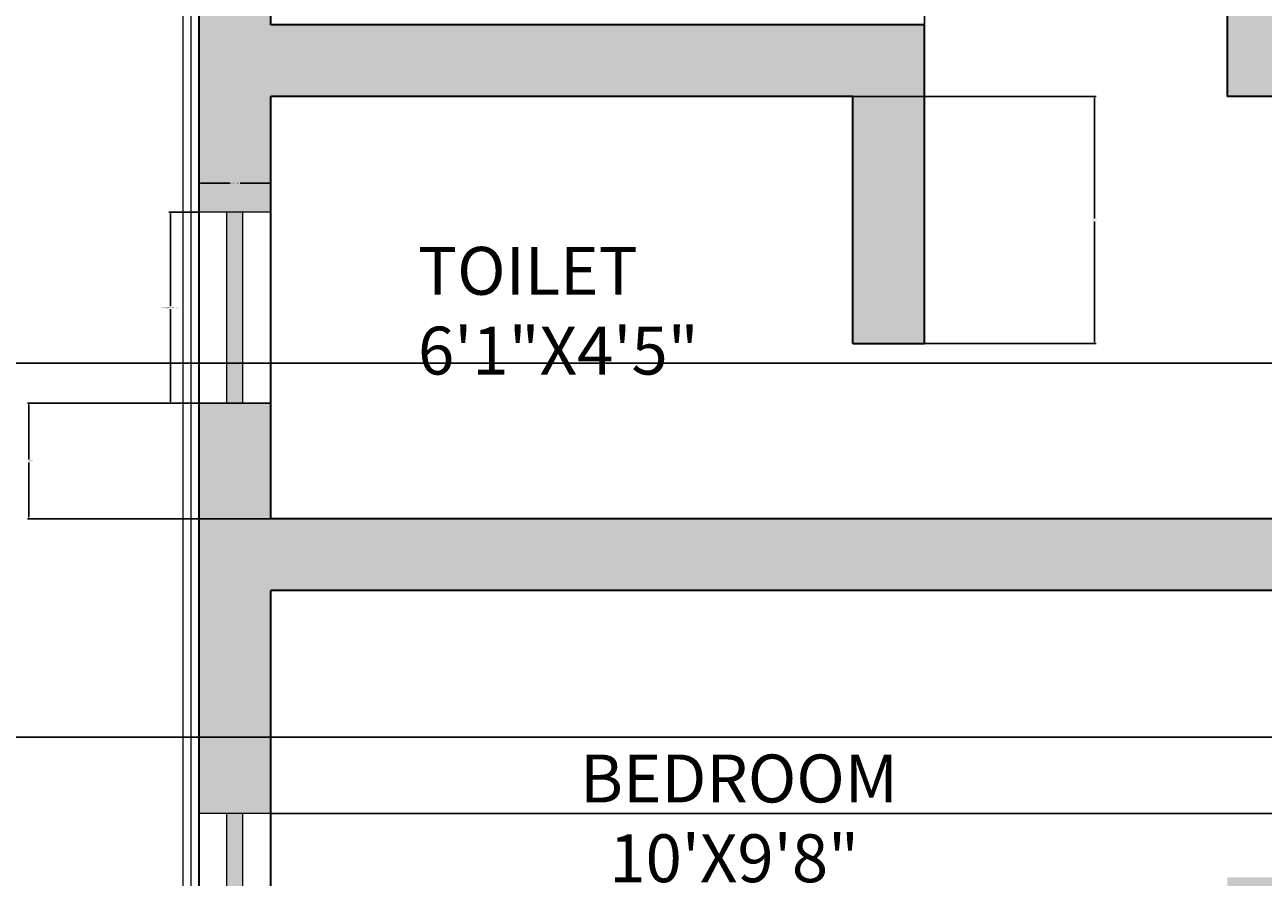
# Model space of a CAD drawing. Units: inches. Extents: x 311 to 815, y -527 to 136.
# Tile 16 of 21: x 388 to 544, y -210 to -103. Entities that reach past the tile are written whole.
import ezdxf

# ---------------------------------------------------------------- set-up
doc = ezdxf.new("R2010")
doc.units = ezdxf.units.IN
doc.header["$MEASUREMENT"] = 0
for name, color, linetype, lineweight in [('A-ANNO-DIMS', 1, 'Continuous', 18), ('A-AREA-IDEN', 8, 'Continuous', 18), ('A-FLOR-EDGE', 1, 'Continuous', 18), ('A-GLAZ-PATT', 5, 'Continuous', 13), ('A-WALL-PATT', 242, 'Continuous', 13), ('wall', 1, 'Continuous', 35), ('win', 5, 'Continuous', 18)]:
    doc.layers.add(name, color=color, linetype=linetype, lineweight=lineweight)
doc.styles.get("Standard").update_dxf_attribs({"font": 'arial.ttf'})
doc.dimstyles.get("Standard").update_dxf_attribs({"dimtxt": 0.18, "dimasz": 0.18, "dimexe": 0.18, "dimexo": 0.0625, "dimgap": 0.09, "dimtad": 0, "dimtih": 1, "dimtoh": 1, "dimdec": 1, "dimzin": 0, "dimdsep": 46, "dimlunit": 4, "dimtxsty": 'Standard', "dimcen": 0.09, "dimadec": 0, "dimazin": 0, "dimtfac": 1, "dimtdec": 1, "dimtofl": 0, "dimtmove": 0, "dimatfit": 3, "dimfxl": 1, "dimtolj": 1, "dimtzin": 0, "dimarcsym": 0})

# ---------------------------------------------------------------- blocks, each defined once
blk = doc.blocks.new('_ArchTick')
at = {"color": 0, "linetype": 'ByBlock', "const_width": 0.15}
blk.add_lwpolyline([(-0.5, -0.5), (0.5, 0.5)], dxfattribs=at)
blk = doc.blocks.new('_Oblique')
at = {"color": 0, "linetype": 'ByBlock', "lineweight": -2}
blk.add_line((-0.5, -0.5), (0.5, 0.5), dxfattribs=at)
blk = doc.blocks.new('*D3')
at = {"layer": 'A-ANNO-DIMS', "color": 0, "lineweight": -2, "transparency": 16777216}
for p, q in [((377.54, 21.87), (377.54, -221.61)), ((377.54, -482.13), (377.54, -238.65))]:
    blk.add_line(p, q, dxfattribs=at)
at = {"layer": 'Defpoints', "color": 0, "transparency": 16777216}
for p in [(410.32, 21.87), (377.54, -482.13), (410.32, -482.13)]:
    blk.add_point(p, dxfattribs=at)
at = {"layer": 'A-ANNO-DIMS', "color": 0, "lineweight": -2, "transparency": 16777216, "xscale": 9, "yscale": 9, "zscale": 9}
for name, p, rotation in [('_ArchTick', (377.54, 21.87), 90), ('_Oblique', (377.54, -482.13), 270)]:
    blk.add_blockref(name, p, dxfattribs=dict(at, rotation=rotation))
at = {"layer": 'A-ANNO-DIMS', "color": 0, "transparency": 16777216, "insert": (377.54, -230.13), "char_height": 9, "attachment_point": 5}
blk.add_mtext("\\A1;42'", dxfattribs=at)
blk = doc.blocks.new('WIN-60IN')
for p, q in [((9, 60), (0, 60)), ((3.5, 0), (3.5, 60)), ((5.5, 0), (5.5, 60)), ((9, 0), (0, 0))]:
    blk.add_line(p, q)
blk = doc.blocks.new('WIN-24IN')
for p, q in [((9, 24), (0, 24)), ((3.5, 0), (3.5, 24)), ((5.5, 0), (5.5, 24)), ((9, 0), (0, 0))]:
    blk.add_line(p, q)
blk = doc.blocks.new('*D12')
at = {"layer": 'A-ANNO-DIMS', "color": 0, "lineweight": -2, "transparency": 16777216}
for p, q in [((410.26, -126.63), (406.54, -126.63)), ((406.72, -126.81), (406.72, -138.44)), ((406.72, -150.45), (406.72, -138.81)), ((410.26, -150.63), (406.54, -150.63))]:
    blk.add_line(p, q, dxfattribs=at)
at = {"layer": 'A-ANNO-DIMS', "color": 0, "transparency": 16777216}
for points in [[(406.69, -126.81), (406.75, -126.81), (406.72, -126.63)], [(406.69, -150.45), (406.75, -150.45), (406.72, -150.63)]]:
    blk.add_solid(points, dxfattribs=at)
at = {"layer": 'Defpoints', "color": 0, "transparency": 16777216}
for p in [(406.72, -126.63), (410.32, -126.63), (410.32, -150.63)]:
    blk.add_point(p, dxfattribs=at)
at = {"layer": 'A-ANNO-DIMS', "color": 0, "transparency": 16777216, "insert": (406.72, -138.63), "char_height": 0.18, "attachment_point": 5}
blk.add_mtext('\\A1;WINDOW 2\'-0" TYP.', dxfattribs=at)
blk = doc.blocks.new('*D13')
at = {"layer": 'A-ANNO-DIMS', "color": 0, "lineweight": -2, "transparency": 16777216}
for p, q in [((410.32, -126.57), (410.32, -122.85)), ((410.5, -123.03), (414.18, -123.03)), ((419.14, -123.03), (415.46, -123.03)), ((419.32, -126.57), (419.32, -122.85))]:
    blk.add_line(p, q, dxfattribs=at)
at = {"layer": 'A-ANNO-DIMS', "color": 0, "transparency": 16777216}
for points in [[(410.5, -123), (410.5, -123.06), (410.32, -123.03)], [(419.14, -123), (419.14, -123.06), (419.32, -123.03)]]:
    blk.add_solid(points, dxfattribs=at)
at = {"layer": 'Defpoints', "color": 0, "transparency": 16777216}
for p in [(419.32, -123.03), (410.32, -126.63), (419.32, -126.63)]:
    blk.add_point(p, dxfattribs=at)
at = {"layer": 'A-ANNO-DIMS', "color": 0, "transparency": 16777216, "insert": (414.82, -123.03), "char_height": 0.18, "attachment_point": 5}
blk.add_mtext('\\A1;0\'-9" TYP.', dxfattribs=at)
blk = doc.blocks.new('*D32')
at = {"layer": 'A-ANNO-DIMS', "color": 0, "lineweight": -2, "transparency": 16777216}
for p, q in [((671.64, -145.62), (377.79, -145.62)), ((377.97, -145.8), (377.97, -168.9)), ((377.97, -192.37), (377.97, -169.27)), ((671.64, -192.55), (377.79, -192.55))]:
    blk.add_line(p, q, dxfattribs=at)
at = {"layer": 'A-ANNO-DIMS', "color": 0, "transparency": 16777216}
for points in [[(377.94, -145.8), (378, -145.8), (377.97, -145.62)], [(377.94, -192.37), (378, -192.37), (377.97, -192.55)]]:
    blk.add_solid(points, dxfattribs=at)
at = {"layer": 'Defpoints', "color": 0, "transparency": 16777216}
for p in [(671.7, -145.62), (377.97, -192.55), (671.7, -192.55)]:
    blk.add_point(p, dxfattribs=at)
at = {"layer": 'A-ANNO-DIMS', "color": 0, "transparency": 16777216, "insert": (377.97, -169.08), "char_height": 0.18, "attachment_point": 5}
blk.add_mtext('\\A1;3\'-11"', dxfattribs=at)
blk = doc.blocks.new('*D41')
at = {"layer": 'A-ANNO-DIMS', "color": 0, "lineweight": -2, "transparency": 16777216}
for p, q in [((419.26, -150.63), (388.79, -150.63)), ((388.97, -150.81), (388.97, -157.69)), ((388.97, -164.95), (388.97, -158.06)), ((419.26, -165.13), (388.79, -165.13))]:
    blk.add_line(p, q, dxfattribs=at)
at = {"layer": 'A-ANNO-DIMS', "color": 0, "transparency": 16777216}
for points in [[(388.94, -150.81), (389, -150.81), (388.97, -150.63)], [(388.94, -164.95), (389, -164.95), (388.97, -165.13)]]:
    blk.add_solid(points, dxfattribs=at)
at = {"layer": 'Defpoints', "color": 0, "transparency": 16777216}
for p in [(388.97, -150.63), (419.32, -150.63), (419.32, -165.13)]:
    blk.add_point(p, dxfattribs=at)
at = {"layer": 'A-ANNO-DIMS', "color": 0, "transparency": 16777216, "insert": (388.97, -157.88), "char_height": 0.18, "attachment_point": 5}
blk.add_mtext('\\A1;1\'-2 1/2"', dxfattribs=at)
blk = doc.blocks.new('*D42')
at = {"layer": 'A-ANNO-DIMS', "color": 0, "lineweight": -2, "transparency": 16777216}
for p, q in [((419.39, -174.13), (754.85, -174.13)), ((754.67, -174.31), (754.67, -187.95)), ((754.67, -201.95), (754.67, -188.31)), ((419.39, -202.13), (754.85, -202.13))]:
    blk.add_line(p, q, dxfattribs=at)
at = {"layer": 'A-ANNO-DIMS', "color": 0, "transparency": 16777216}
for points in [[(754.64, -174.31), (754.7, -174.31), (754.67, -174.13)], [(754.64, -201.95), (754.7, -201.95), (754.67, -202.13)]]:
    blk.add_solid(points, dxfattribs=at)
at = {"layer": 'Defpoints', "color": 0, "transparency": 16777216}
for p in [(419.32, -174.13), (419.32, -202.13), (754.67, -202.13)]:
    blk.add_point(p, dxfattribs=at)
at = {"layer": 'A-ANNO-DIMS', "color": 0, "transparency": 16777216, "insert": (754.67, -188.13), "char_height": 0.18, "attachment_point": 5}
blk.add_mtext('\\A1;2\'-4"', dxfattribs=at)
blk = doc.blocks.new('*D51')
at = {"layer": 'A-ANNO-DIMS', "color": 0, "lineweight": -2, "transparency": 16777216}
for p, q in [((501.32, -103.07), (501.32, 54.4)), ((539.32, -112.07), (539.32, 54.4)), ((501.5, 54.22), (519.99, 54.22)), ((539.14, 54.22), (520.65, 54.22))]:
    blk.add_line(p, q, dxfattribs=at)
at = {"layer": 'A-ANNO-DIMS', "color": 0, "transparency": 16777216}
for points in [[(501.5, 54.25), (501.5, 54.19), (501.32, 54.22)], [(539.14, 54.25), (539.14, 54.19), (539.32, 54.22)]]:
    blk.add_solid(points, dxfattribs=at)
at = {"layer": 'Defpoints', "color": 0, "transparency": 16777216}
for p in [(501.32, 54.22), (501.32, -103.13), (539.32, -112.13)]:
    blk.add_point(p, dxfattribs=at)
at = {"layer": 'A-ANNO-DIMS', "color": 0, "transparency": 16777216, "insert": (520.32, 54.22), "char_height": 0.18, "attachment_point": 5}
blk.add_mtext('\\A1;3\'-2"', dxfattribs=at)
blk = doc.blocks.new('*D55')
at = {"layer": 'A-ANNO-DIMS', "color": 0, "lineweight": -2, "transparency": 16777216}
for p, q in [((492.39, -112.13), (522.85, -112.13)), ((522.67, -112.31), (522.67, -127.45)), ((522.67, -142.95), (522.67, -127.81)), ((492.39, -143.13), (522.85, -143.13))]:
    blk.add_line(p, q, dxfattribs=at)
at = {"layer": 'A-ANNO-DIMS', "color": 0, "transparency": 16777216}
for points in [[(522.64, -112.31), (522.7, -112.31), (522.67, -112.13)], [(522.64, -142.95), (522.7, -142.95), (522.67, -143.13)]]:
    blk.add_solid(points, dxfattribs=at)
at = {"layer": 'Defpoints', "color": 0, "transparency": 16777216}
for p in [(492.32, -112.13), (492.32, -143.13), (522.67, -143.13)]:
    blk.add_point(p, dxfattribs=at)
at = {"layer": 'A-ANNO-DIMS', "color": 0, "transparency": 16777216, "insert": (522.67, -127.63), "char_height": 0.18, "attachment_point": 5}
blk.add_mtext('\\A1;2\'-7"', dxfattribs=at)

msp = doc.modelspace()

# ---------------------------------------------------------------- hatches: boundary and pattern name
at = {"layer": 'A-GLAZ-PATT'}
h = msp.add_hatch(color=256, dxfattribs=at)
h.dxf.hatch_style = 1
h.paths.add_polyline_path([(415.82, -202.13), (413.82, -202.13), (413.82, -262.13), (415.82, -262.13)])
h.paths.add_polyline_path([(415.82, -390.84), (413.82, -390.84), (413.82, -450.84), (415.82, -450.84)])
h.paths.add_polyline_path([(415.82, -311.57), (413.82, -311.57), (413.82, -335.57), (415.82, -335.57)])
h.paths.add_polyline_path([(509.32, -476.63), (449.32, -476.63), (449.32, -478.63), (509.32, -478.63)])
h.paths.add_polyline_path([(606.82, -476.63), (582.82, -476.63), (582.82, -478.63), (606.82, -478.63)])
h.paths.add_polyline_path([(678.82, -476.63), (654.82, -476.63), (654.82, -478.63), (678.82, -478.63)])
h.paths.add_polyline_path([(718.82, -385.13), (716.82, -385.13), (716.82, -445.13), (718.82, -445.13)])
h.paths.add_polyline_path([(718.82, -262.63), (716.82, -262.63), (716.82, -322.63), (718.82, -322.63)])
h.paths.add_polyline_path([(718.82, -140.13), (716.82, -140.13), (716.82, -200.13), (718.82, -200.13)])
h.paths.add_polyline_path([(718.82, -18.13), (716.82, -18.13), (716.82, -42.13), (718.82, -42.13)])
h.paths.add_polyline_path([(686.82, 18.37), (626.82, 18.37), (626.82, 16.37), (686.82, 16.37)])
h.paths.add_polyline_path([(581.82, 18.37), (557.82, 18.37), (557.82, 16.37), (581.82, 16.37)])
h.paths.add_polyline_path([(509.32, 18.37), (449.32, 18.37), (449.32, 16.37), (509.32, 16.37)])
h = msp.add_hatch(color=256, dxfattribs=at)
h.dxf.hatch_style = 1
h.paths.add_polyline_path([(415.82, -15.13), (413.82, -15.13), (413.82, -75.13), (415.82, -75.13)])
h.paths.add_polyline_path([(415.82, -126.63), (413.82, -126.63), (413.82, -150.63), (415.82, -150.63)])
at = {"layer": 'A-WALL-PATT'}
h = msp.add_hatch(color=256, dxfattribs=at)
h.dxf.hatch_style = 1
h.paths.add_polyline_path([(557.82, 21.87), (509.32, 21.87), (509.32, 12.87), (539.32, 12.87), (539.32, -112.13), (548.32, -112.13), (548.32, -58.63), (557.82, -58.63), (557.82, -49.63), (548.32, -49.63), (548.32, 12.87), (557.82, 12.87)])
h.paths.add_polyline_path([(449.32, 21.87), (410.32, 21.87), (410.32, -15.13), (419.32, -15.13), (419.32, 12.87), (449.32, 12.87)])
h.paths.add_polyline_path([(626.82, 21.87), (581.82, 21.87), (581.82, 12.87), (591.32, 12.87), (591.32, -49.63), (581.82, -49.63), (581.82, -58.63), (591.32, -58.63), (591.32, -112.13), (600.32, -112.13), (600.32, 12.87), (626.82, 12.87)])
h.paths.add_polyline_path([(722.32, 21.87), (686.82, 21.87), (686.82, 12.87), (713.32, 12.87), (713.32, -18.13), (722.32, -18.13)])
h.paths.add_polyline_path([(722.32, -42.13), (713.32, -42.13), (713.32, -73.13), (722.32, -73.13)])
h.paths.add_polyline_path([(501.32, -103.13), (419.32, -103.13), (419.32, -75.13), (410.32, -75.13), (410.32, -126.63), (419.32, -126.63), (419.32, -112.13), (492.32, -112.13), (492.32, -143.13), (501.32, -143.13)])
h.paths.add_polyline_path([(548.32, -165.13), (419.32, -165.13), (419.32, -150.63), (410.32, -150.63), (410.32, -202.13), (419.32, -202.13), (419.32, -174.13), (548.32, -174.13)])
h.paths.add_polyline_path([(722.32, -103.13), (636.32, -103.13), (636.32, -112.13), (713.32, -112.13), (713.32, -140.13), (722.32, -140.13)])
h.paths.add_polyline_path([(548.32, -210.13), (539.32, -210.13), (539.32, -290.13), (419.32, -290.13), (419.32, -262.13), (410.32, -262.13), (410.32, -311.57), (419.32, -311.57), (419.32, -299.13), (469.32, -299.13), (469.32, -348.13), (443.32, -348.13), (443.32, -357.13), (478.32, -357.13), (478.32, -299.13), (548.32, -299.13)])
h.paths.add_polyline_path([(722.32, -200.13), (713.32, -200.13), (713.32, -228.13), (609.32, -228.13), (609.32, -237.13), (713.32, -237.13), (713.32, -262.63), (722.32, -262.63)])
h.paths.add_polyline_path([(722.32, -322.63), (713.32, -322.63), (713.32, -348.13), (633.32, -348.13), (633.32, -357.13), (713.32, -357.13), (713.32, -385.13), (722.32, -385.13)])
h.paths.add_polyline_path([(419.32, -335.57), (410.32, -335.57), (410.32, -390.84), (419.32, -390.84)])
h.paths.add_polyline_path([(419.32, -450.84), (410.32, -450.84), (410.32, -482.13), (449.32, -482.13), (449.32, -473.13), (419.32, -473.13)])
h.paths.add_polyline_path([(582.82, -473.13), (548.32, -473.13), (548.32, -348.13), (539.32, -348.13), (539.32, -473.13), (509.32, -473.13), (509.32, -482.13), (582.82, -482.13)])
h.paths.add_polyline_path([(722.32, -445.13), (713.32, -445.13), (713.32, -473.13), (678.82, -473.13), (678.82, -482.13), (722.32, -482.13)])

# ---------------------------------------------------------------- linework, layer by layer
at = {"layer": 'A-FLOR-EDGE'}
for p, q in [((408.32, -484.13), (408.32, 23.87)), ((409.32, -483.13), (409.32, 22.87))]:
    msp.add_line(p, q, dxfattribs=at)
at = {"layer": 'wall'}
for p, q in [((410.32, -482.13), (410.32, 21.87)), ((419.32, -103.13), (419.32, 12.87)), ((539.32, -112.13), (539.32, 12.87)), ((539.32, -112.13), (539.32, 12.87)), ((501.32, -103.13), (419.32, -103.13)), ((501.32, -143.13), (501.32, -103.13)), ((492.32, -112.13), (419.32, -112.13)), ((419.32, -165.13), (419.32, -112.13)), ((492.32, -143.13), (492.32, -112.13)), ((548.32, -112.13), (539.32, -112.13)), ((492.32, -143.13), (501.32, -143.13)), ((548.32, -165.13), (419.32, -165.13)), ((548.32, -174.13), (419.32, -174.13)), ((419.32, -290.13), (419.32, -174.13))]:
    msp.add_line(p, q, dxfattribs=at)

# ---------------------------------------------------------------- block references
at = {"layer": 'win'}
for name, p in [('WIN-24IN', (410.32, -150.63)), ('WIN-60IN', (410.32, -262.13))]:
    msp.add_blockref(name, p, dxfattribs=at)

# ---------------------------------------------------------------- texts
at = {"layer": 'A-AREA-IDEN', "char_height": 6.0073, "attachment_point": 1}
for s, width, insert in [('    TOILET\\P    6\'1"X4\'5"', 47.2824, (430.44, -131.01)), ('    BEDROOM\\P      10\'X9\'8"', 59.0599, (450.77, -194.73))]:
    msp.add_mtext_dynamic_manual_height_columns(s, width=width, gutter_width=1, heights=[0], dxfattribs=dict(at, insert=insert))

# ---------------------------------------------------------------- dimensions: what is measured, and where the dimension line sits
at = {"layer": 'A-ANNO-DIMS'}
dim = msp.add_linear_dim(base=(501.32, 54.22), p1=(539.32, -112.13), p2=(501.32, -103.13), dimstyle='Standard', override={"dimdec": 1, "dimlfac": 1, "dimrnd": 0, "dimzin": 1, "dimdsep": 46, "dimlunit": 4, "dimfrac": 2}, dxfattribs=at)
dim.commit()
dim.dimension.update_dxf_attribs({"geometry": '*D51', "text_midpoint": (520.32, 54.22)})
for base, p1, p2, angle, override, picture, middle in [((377.54, -482.13), (410.32, 21.87), (410.32, -482.13), 90, {"dimtxt": 9, "dimasz": 9, "dimgap": 4, "dimblk1": 'ArchTick', "dimblk2": 'Oblique', "dimsah": 1, "dimse1": 1, "dimse2": 1, "dimclrd": 0, "dimclre": 0, "dimclrt": 0}, '*D3', (377.54, -230.13)), ((522.67, -143.13), (492.32, -112.13), (492.32, -143.13), 270, {"dimdec": 1, "dimlfac": 1, "dimrnd": 0, "dimzin": 1, "dimdsep": 46, "dimlunit": 4, "dimfrac": 2}, '*D55', (522.67, -127.63)), ((377.97, -192.55), (671.7, -145.62), (671.7, -192.55), 90, {"dimdec": 1, "dimlfac": 1, "dimrnd": 0, "dimzin": 1, "dimdsep": 46, "dimlunit": 4, "dimfrac": 2}, '*D32', (377.97, -169.08)), ((388.97, -150.63), (419.32, -165.13), (419.32, -150.63), 90, {"dimdec": 1, "dimlfac": 1, "dimrnd": 0, "dimzin": 1, "dimdsep": 46, "dimlunit": 4, "dimfrac": 2}, '*D41', (388.97, -157.88)), ((754.67, -202.13), (419.32, -174.13), (419.32, -202.13), 90, {"dimdec": 1, "dimlfac": 1, "dimrnd": 0, "dimzin": 1, "dimdsep": 46, "dimlunit": 4, "dimfrac": 2}, '*D42', (754.67, -188.13))]:
    dim = msp.add_linear_dim(base=base, p1=p1, p2=p2, angle=angle, dimstyle='Standard', override=override, dxfattribs=at)
    dim.commit()
    dim.dimension.update_dxf_attribs({"geometry": picture, "text_midpoint": middle})
dim = msp.add_linear_dim(base=(419.32, -123.03), p1=(410.32, -126.63), p2=(419.32, -126.63), text='<> TYP.', dimstyle='Standard', override={"dimdec": 1, "dimlfac": 1, "dimrnd": 0, "dimzin": 1, "dimdsep": 46, "dimlunit": 4, "dimfrac": 2}, dxfattribs=at)
dim.commit()
dim.dimension.update_dxf_attribs({"geometry": '*D13', "text_midpoint": (414.82, -123.03)})
dim = msp.add_linear_dim(base=(406.72, -126.63), p1=(410.32, -150.63), p2=(410.32, -126.63), angle=90, text='WINDOW <> TYP.', dimstyle='Standard', override={"dimdec": 1, "dimlfac": 1, "dimrnd": 0, "dimzin": 1, "dimdsep": 46, "dimlunit": 4, "dimfrac": 2}, dxfattribs=at)
dim.commit()
dim.dimension.update_dxf_attribs({"geometry": '*D12', "text_midpoint": (406.72, -138.63)})

doc.saveas('drawing.dxf')
